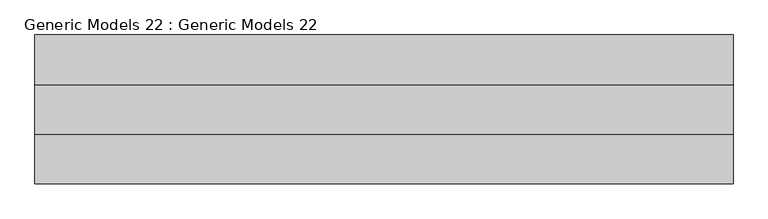
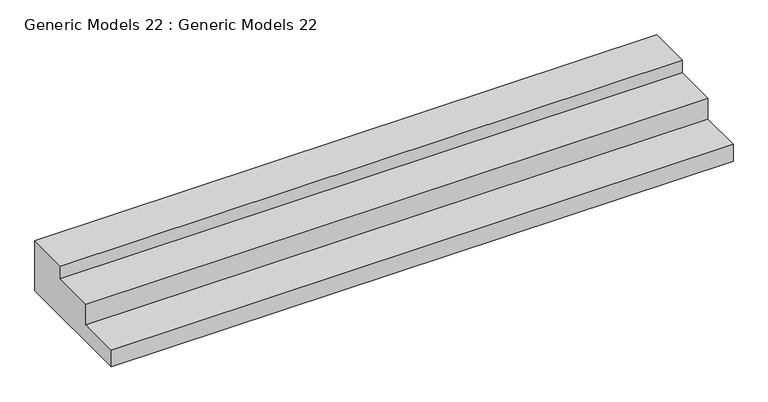
"""IFC4 building model written with IfcOpenShell, lengths in millimetres: proxy geometry, Generic Models 22 : Generic Models 22."""

from ifc_helpers import new_model, si_unit, frame, origin, place, context, project, spatial, polyline, outline, extrude, source, transform, mapped, element, save


def generic_models_22_generic_models_22_fd5cddf6(model_context):
    return source(origin(), model_context, "Body", "SweptSolid", [
        extrude(outline(polyline([(-9574.3210084, 0.0), (-10336.3210084, 0.0), (-10336.3210084, 101.6), (-10082.3210084, 101.6), (-10082.3210084, 228.6), (-9828.3210084, 228.6), (-9828.3210084, 304.8), (-9574.3210084, 304.8), (-9574.3210084, 0.0)])), frame((-9891.8681672, 0.0, 0.0), z_axis=(1.0, 0.0, 0.0), x_axis=(0.0, 1.0, 0.0)), (0.0, 0.0, 1.0), 3571.9350882),
    ])


if __name__ == "__main__":
    model = new_model("IFC4")
    model_context = context("Model", 3, world=origin())
    ifc_project = project(units=[si_unit("LENGTHUNIT", "METRE", prefix="MILLI")], contexts=[model_context])
    site = spatial("IfcSite", under=ifc_project)
    building = spatial("IfcBuilding", under=site)
    placement = place(None, origin())
    generic_models_22_generic_models_22_shape = generic_models_22_generic_models_22_fd5cddf6(model_context)
    element("IfcBuildingElementProxy", 1, Name="Generic Models 22 : Generic Models 22", ObjectType="Generic Models 22 : Generic Models 22", at=placement, inside=building, context=model_context, shape_type="MappedRepresentation", body=[
        mapped(generic_models_22_generic_models_22_shape, transform((0.0, 0.0, 0.0), x_axis=(1.0, 0.0, 0.0), y_axis=(0.0, 1.0, 0.0), z_axis=(0.0, 0.0, 1.0))),
    ])
    save(model, "model.ifc")

# Revit data of these elements
# Element 1 (IfcBuildingElementProxy, "Generic Models 22 : Generic Models 22")
#   Materials on its faces: "CAST IN PLACE STAIRS"
# Materials
#   "CAST IN PLACE STAIRS": class "Generic", colour RGB 120 120 120, transparency 0, Cost = 0
